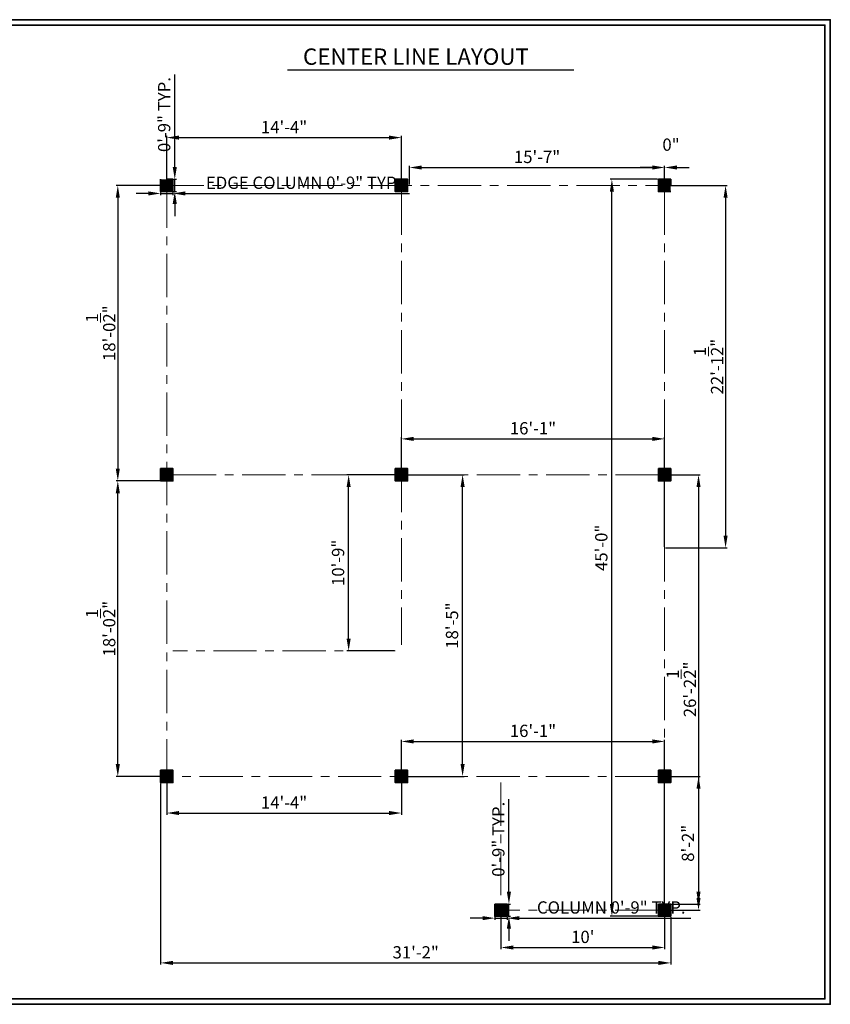
# Model space of a CAD drawing. Units: inches. Extents: x 2396 to 4051, y 1419 to 2191.
# Tile 7 of 7: x 3457 to 4051, y 1470 to 2191. Entities that reach past the tile are written whole.
import ezdxf

# ---------------------------------------------------------------- set-up
doc = ezdxf.new("R2010")
doc.units = ezdxf.units.IN
doc.linetypes.add('CENTER', pattern=[50.8, 31.75, -6.35, 6.35, -6.35])
for name, color, linetype, lineweight in [('A-ANNO-TITL', 7, 'Continuous', 25), ('A-ANNO-TTLB', 7, 'Continuous', 35), ('S-ANNO-DIMS', 2, 'Continuous', 18), ('S-GRID', 1, 'CENTER', 18)]:
    doc.layers.add(name, color=color, linetype=linetype, lineweight=lineweight)
doc.layers.add('S-COLS', color=242, linetype='Continuous', lineweight=35, true_color=0xcd2027)
doc.styles.get("Standard").update_dxf_attribs({"font": 'arial.ttf'})
doc.dimstyles.new('ISO-25', dxfattribs={"dimtxt": 9, "dimasz": 9, "dimexe": 1.25, "dimexo": 0.625, "dimgap": 2, "dimtad": 1, "dimdec": 1, "dimlunit": 4, "dimtxsty": 'Standard', "dimcen": 2.5, "dimadec": 0, "dimazin": 0, "dimtfac": 1, "dimtdec": 1, "dimtmove": 0, "dimatfit": 3, "dimfxl": 1, "dimarcsym": 0})

# ---------------------------------------------------------------- blocks, each defined once
blk = doc.blocks.new('*D15')
at = {"layer": 'Defpoints', "color": 0, "transparency": 16777216}
for p in [(3736.71, 2104.86), (3564.71, 2069.8), (3736.71, 2069.8)]:
    blk.add_point(p, dxfattribs=at)
at = {"layer": 'S-ANNO-DIMS', "color": 0, "lineweight": -2, "transparency": 16777216}
for p, q in [((3564.71, 2070.43), (3564.71, 2106.11)), ((3573.71, 2104.86), (3727.71, 2104.86)), ((3736.71, 2070.43), (3736.71, 2106.11))]:
    blk.add_line(p, q, dxfattribs=at)
at = {"layer": 'S-ANNO-DIMS', "color": 0, "transparency": 16777216}
for points in [[(3573.71, 2106.36), (3573.71, 2103.36), (3564.71, 2104.86)], [(3727.71, 2106.36), (3727.71, 2103.36), (3736.71, 2104.86)]]:
    blk.add_solid(points, dxfattribs=at)
at = {"layer": 'S-ANNO-DIMS', "color": 0, "transparency": 16777216, "insert": (3650.71, 2111.38), "char_height": 9, "attachment_point": 5}
blk.add_mtext('14\'-4"', dxfattribs=at)
blk = doc.blocks.new('*D16')
at = {"layer": 'Defpoints', "color": 0, "transparency": 16777216}
for p in [(3929.71, 2082.95), (3742.71, 2069.8), (3929.71, 2069.8)]:
    blk.add_point(p, dxfattribs=at)
at = {"layer": 'S-ANNO-DIMS', "color": 0, "lineweight": -2, "transparency": 16777216}
for p, q in [((3742.71, 2070.43), (3742.71, 2084.2)), ((3751.71, 2082.95), (3920.71, 2082.95)), ((3929.71, 2070.43), (3929.71, 2084.2))]:
    blk.add_line(p, q, dxfattribs=at)
at = {"layer": 'S-ANNO-DIMS', "color": 0, "transparency": 16777216}
for points in [[(3751.71, 2084.45), (3751.71, 2081.45), (3742.71, 2082.95)], [(3920.71, 2084.45), (3920.71, 2081.45), (3929.71, 2082.95)]]:
    blk.add_solid(points, dxfattribs=at)
at = {"layer": 'S-ANNO-DIMS', "color": 0, "transparency": 16777216, "insert": (3836.21, 2089.54), "char_height": 9, "attachment_point": 5}
blk.add_mtext('15\'-7"', dxfattribs=at)
blk = doc.blocks.new('*D17')
at = {"layer": 'Defpoints', "color": 0, "transparency": 16777216}
for p in [(3929.71, 2082.95), (3929.71, 2082.95), (3929.71, 2069.8)]:
    blk.add_point(p, dxfattribs=at)
at = {"layer": 'S-ANNO-DIMS', "color": 0, "lineweight": -2, "transparency": 16777216}
for p, q in [((3920.71, 2082.95), (3911.71, 2082.95)), ((3929.71, 2070.43), (3929.71, 2084.2)), ((3929.71, 2083.57), (3929.71, 2084.2)), ((3938.71, 2082.95), (3947.71, 2082.95))]:
    blk.add_line(p, q, dxfattribs=at)
at = {"layer": 'S-ANNO-DIMS', "color": 0, "transparency": 16777216}
for points in [[(3920.71, 2084.45), (3920.71, 2081.45), (3929.71, 2082.95)], [(3938.71, 2084.45), (3938.71, 2081.45), (3929.71, 2082.95)]]:
    blk.add_solid(points, dxfattribs=at)
at = {"layer": 'S-ANNO-DIMS', "color": 0, "transparency": 16777216, "insert": (3934.41, 2098.54), "char_height": 9, "attachment_point": 5}
blk.add_mtext('0"', dxfattribs=at)
blk = doc.blocks.new('*D18')
at = {"layer": 'Defpoints', "color": 0, "transparency": 16777216}
for p in [(3564.71, 2069.8), (3528.81, 1853.3), (3564.71, 1853.3)]:
    blk.add_point(p, dxfattribs=at)
at = {"layer": 'S-ANNO-DIMS', "color": 0, "lineweight": -2, "transparency": 16777216}
for p, q in [((3564.09, 2069.8), (3527.56, 2069.8)), ((3528.81, 2060.8), (3528.81, 1862.3)), ((3564.09, 1853.3), (3527.56, 1853.3))]:
    blk.add_line(p, q, dxfattribs=at)
at = {"layer": 'S-ANNO-DIMS', "color": 0, "transparency": 16777216}
for points in [[(3527.31, 2060.8), (3530.31, 2060.8), (3528.81, 2069.8)], [(3527.31, 1862.3), (3530.31, 1862.3), (3528.81, 1853.3)]]:
    blk.add_solid(points, dxfattribs=at)
at = {"layer": 'S-ANNO-DIMS', "color": 0, "transparency": 16777216, "insert": (3516.2, 1961.55), "char_height": 9, "attachment_point": 5, "rotation": 90}
blk.add_mtext('18\'-0{\\H1x;\\S1/2;}"', dxfattribs=at)
blk = doc.blocks.new('*D19')
at = {"layer": 'Defpoints', "color": 0, "transparency": 16777216}
for p in [(3528.81, 1853.3), (3564.71, 1853.3), (3564.71, 1636.8)]:
    blk.add_point(p, dxfattribs=at)
at = {"layer": 'S-ANNO-DIMS', "color": 0, "lineweight": -2, "transparency": 16777216}
for p, q in [((3564.09, 1853.3), (3527.56, 1853.3)), ((3528.81, 1645.8), (3528.81, 1844.3)), ((3564.09, 1636.8), (3527.56, 1636.8))]:
    blk.add_line(p, q, dxfattribs=at)
at = {"layer": 'S-ANNO-DIMS', "color": 0, "transparency": 16777216}
for points in [[(3527.31, 1844.3), (3530.31, 1844.3), (3528.81, 1853.3)], [(3527.31, 1645.8), (3530.31, 1645.8), (3528.81, 1636.8)]]:
    blk.add_solid(points, dxfattribs=at)
at = {"layer": 'S-ANNO-DIMS', "color": 0, "transparency": 16777216, "insert": (3516.2, 1745.05), "char_height": 9, "attachment_point": 5, "rotation": 90}
blk.add_mtext('18\'-0{\\H1x;\\S1/2;}"', dxfattribs=at)
blk = doc.blocks.new('*D20')
at = {"layer": 'Defpoints', "color": 0, "transparency": 16777216}
for p in [(3564.71, 1632.3), (3736.71, 1636.8), (3736.71, 1609.97)]:
    blk.add_point(p, dxfattribs=at)
at = {"layer": 'S-ANNO-DIMS', "color": 0, "lineweight": -2, "transparency": 16777216}
for p, q in [((3564.71, 1631.68), (3564.71, 1608.72)), ((3736.71, 1636.18), (3736.71, 1608.72)), ((3573.71, 1609.97), (3727.71, 1609.97))]:
    blk.add_line(p, q, dxfattribs=at)
at = {"layer": 'S-ANNO-DIMS', "color": 0, "transparency": 16777216}
for points in [[(3573.71, 1611.47), (3573.71, 1608.47), (3564.71, 1609.97)], [(3727.71, 1611.47), (3727.71, 1608.47), (3736.71, 1609.97)]]:
    blk.add_solid(points, dxfattribs=at)
at = {"layer": 'S-ANNO-DIMS', "color": 0, "transparency": 16777216, "insert": (3650.71, 1616.49), "char_height": 9, "attachment_point": 5}
blk.add_mtext('14\'-4"', dxfattribs=at)
blk = doc.blocks.new('*D21')
at = {"layer": 'Defpoints', "color": 0, "transparency": 16777216}
for p in [(3929.71, 1662.41), (3736.71, 1636.8), (3929.71, 1543.3)]:
    blk.add_point(p, dxfattribs=at)
at = {"layer": 'S-ANNO-DIMS', "color": 0, "lineweight": -2, "transparency": 16777216}
for p, q in [((3736.71, 1637.43), (3736.71, 1663.66)), ((3745.71, 1662.41), (3920.71, 1662.41)), ((3929.71, 1543.93), (3929.71, 1663.66))]:
    blk.add_line(p, q, dxfattribs=at)
at = {"layer": 'S-ANNO-DIMS', "color": 0, "transparency": 16777216}
for points in [[(3745.71, 1663.91), (3745.71, 1660.91), (3736.71, 1662.41)], [(3920.71, 1663.91), (3920.71, 1660.91), (3929.71, 1662.41)]]:
    blk.add_solid(points, dxfattribs=at)
at = {"layer": 'S-ANNO-DIMS', "color": 0, "transparency": 16777216, "insert": (3833.21, 1669), "char_height": 9, "attachment_point": 5}
blk.add_mtext('16\'-1"', dxfattribs=at)
blk = doc.blocks.new('*D22')
at = {"layer": 'Defpoints', "color": 0, "transparency": 16777216}
for p in [(3929.71, 1636.8), (3929.71, 1538.8), (3954.57, 1538.8)]:
    blk.add_point(p, dxfattribs=at)
at = {"layer": 'S-ANNO-DIMS', "color": 0, "lineweight": -2, "transparency": 16777216}
for p, q in [((3930.34, 1636.8), (3955.82, 1636.8)), ((3954.57, 1627.8), (3954.57, 1547.8)), ((3930.34, 1538.8), (3955.82, 1538.8))]:
    blk.add_line(p, q, dxfattribs=at)
at = {"layer": 'S-ANNO-DIMS', "color": 0, "transparency": 16777216}
for points in [[(3953.07, 1627.8), (3956.07, 1627.8), (3954.57, 1636.8)], [(3953.07, 1547.8), (3956.07, 1547.8), (3954.57, 1538.8)]]:
    blk.add_solid(points, dxfattribs=at)
at = {"layer": 'S-ANNO-DIMS', "color": 0, "transparency": 16777216, "insert": (3947.97, 1587.8), "char_height": 9, "attachment_point": 5, "rotation": 90}
blk.add_mtext('8\'-2"', dxfattribs=at)
blk = doc.blocks.new('*D23')
at = {"layer": 'Defpoints', "color": 0, "transparency": 16777216}
for p in [(3809.71, 1538.8), (3929.71, 1538.8), (3929.71, 1511.44)]:
    blk.add_point(p, dxfattribs=at)
at = {"layer": 'S-ANNO-DIMS', "color": 0, "lineweight": -2, "transparency": 16777216}
for p, q in [((3809.71, 1538.18), (3809.71, 1510.19)), ((3929.71, 1538.18), (3929.71, 1510.19)), ((3818.71, 1511.44), (3920.71, 1511.44))]:
    blk.add_line(p, q, dxfattribs=at)
at = {"layer": 'S-ANNO-DIMS', "color": 0, "transparency": 16777216}
for points in [[(3818.71, 1512.94), (3818.71, 1509.94), (3809.71, 1511.44)], [(3920.71, 1512.94), (3920.71, 1509.94), (3929.71, 1511.44)]]:
    blk.add_solid(points, dxfattribs=at)
at = {"layer": 'S-ANNO-DIMS', "color": 0, "transparency": 16777216, "insert": (3869.71, 1518.04), "char_height": 9, "attachment_point": 5}
blk.add_mtext("10'", dxfattribs=at)
blk = doc.blocks.new('*D24')
at = {"layer": 'Defpoints', "color": 0, "transparency": 16777216}
for p in [(3929.71, 2069.8), (3929.71, 1804.3), (3974.42, 1804.3)]:
    blk.add_point(p, dxfattribs=at)
at = {"layer": 'S-ANNO-DIMS', "color": 0, "lineweight": -2, "transparency": 16777216}
for p, q in [((3930.34, 2069.8), (3975.67, 2069.8)), ((3974.42, 2060.8), (3974.42, 1813.3)), ((3930.34, 1804.3), (3975.67, 1804.3))]:
    blk.add_line(p, q, dxfattribs=at)
at = {"layer": 'S-ANNO-DIMS', "color": 0, "transparency": 16777216}
for points in [[(3972.92, 2060.8), (3975.92, 2060.8), (3974.42, 2069.8)], [(3972.92, 1813.3), (3975.92, 1813.3), (3974.42, 1804.3)]]:
    blk.add_solid(points, dxfattribs=at)
at = {"layer": 'S-ANNO-DIMS', "color": 0, "transparency": 16777216, "insert": (3961.89, 1937.05), "char_height": 9, "attachment_point": 5, "rotation": 90}
blk.add_mtext('22\'-1{\\H1x;\\S1/2;}"', dxfattribs=at)
blk = doc.blocks.new('*D25')
at = {"layer": 'Defpoints', "color": 0, "transparency": 16777216}
for p in [(3929.71, 1857.8), (3929.71, 1543.3), (3954.57, 1543.3)]:
    blk.add_point(p, dxfattribs=at)
at = {"layer": 'S-ANNO-DIMS', "color": 0, "lineweight": -2, "transparency": 16777216}
for p, q in [((3930.34, 1857.8), (3955.82, 1857.8)), ((3954.57, 1848.8), (3954.57, 1552.3)), ((3930.34, 1543.3), (3955.82, 1543.3))]:
    blk.add_line(p, q, dxfattribs=at)
at = {"layer": 'S-ANNO-DIMS', "color": 0, "transparency": 16777216}
for points in [[(3953.07, 1848.8), (3956.07, 1848.8), (3954.57, 1857.8)], [(3953.07, 1552.3), (3956.07, 1552.3), (3954.57, 1543.3)]]:
    blk.add_solid(points, dxfattribs=at)
at = {"layer": 'S-ANNO-DIMS', "color": 0, "transparency": 16777216, "insert": (3941.95, 1700.55), "char_height": 9, "attachment_point": 5, "rotation": 90}
blk.add_mtext('26\'-2{\\H1x;\\S1/2;}"', dxfattribs=at)
blk = doc.blocks.new('*D26')
at = {"layer": 'Defpoints', "color": 0, "transparency": 16777216}
for p in [(3929.71, 1884.11), (3736.71, 1857.8), (3929.71, 1804.3)]:
    blk.add_point(p, dxfattribs=at)
at = {"layer": 'S-ANNO-DIMS', "color": 0, "lineweight": -2, "transparency": 16777216}
for p, q in [((3736.71, 1858.43), (3736.71, 1885.36)), ((3745.71, 1884.11), (3920.71, 1884.11)), ((3929.71, 1804.93), (3929.71, 1885.36))]:
    blk.add_line(p, q, dxfattribs=at)
at = {"layer": 'S-ANNO-DIMS', "color": 0, "transparency": 16777216}
for points in [[(3745.71, 1885.61), (3745.71, 1882.61), (3736.71, 1884.11)], [(3920.71, 1885.61), (3920.71, 1882.61), (3929.71, 1884.11)]]:
    blk.add_solid(points, dxfattribs=at)
at = {"layer": 'S-ANNO-DIMS', "color": 0, "transparency": 16777216, "insert": (3833.21, 1890.71), "char_height": 9, "attachment_point": 5}
blk.add_mtext('16\'-1"', dxfattribs=at)
blk = doc.blocks.new('*D27')
at = {"layer": 'Defpoints', "color": 0, "transparency": 16777216}
for p in [(3736.71, 1857.8), (3781.61, 1857.8), (3736.71, 1636.8)]:
    blk.add_point(p, dxfattribs=at)
at = {"layer": 'S-ANNO-DIMS', "color": 0, "lineweight": -2, "transparency": 16777216}
for p, q in [((3737.34, 1857.8), (3782.86, 1857.8)), ((3781.61, 1645.8), (3781.61, 1848.8)), ((3737.34, 1636.8), (3782.86, 1636.8))]:
    blk.add_line(p, q, dxfattribs=at)
at = {"layer": 'S-ANNO-DIMS', "color": 0, "transparency": 16777216}
for points in [[(3780.11, 1848.8), (3783.11, 1848.8), (3781.61, 1857.8)], [(3780.11, 1645.8), (3783.11, 1645.8), (3781.61, 1636.8)]]:
    blk.add_solid(points, dxfattribs=at)
at = {"layer": 'S-ANNO-DIMS', "color": 0, "transparency": 16777216, "insert": (3775.01, 1747.3), "char_height": 9, "attachment_point": 5, "rotation": 90}
blk.add_mtext('18\'-5"', dxfattribs=at)
blk = doc.blocks.new('COL-9X9')
h = blk.add_hatch(color=256)
h.dxf.hatch_style = 1
h.paths.add_polyline_path([(9, 9), (0, 9), (0, 0), (9, 0)])
blk.add_lwpolyline([(0, 9), (9, 9), (9, 0), (0, 0)], close=True)
blk = doc.blocks.new('COL-9X9-EDGE-NODE')
h = blk.add_hatch(color=256)
h.dxf.hatch_style = 1
h.paths.add_polyline_path([(0, 0), (9, 0), (9, 9), (0, 9)])
blk.add_lwpolyline([(4.5, 9), (9, 9), (9, 0), (0, 0), (0, 9)])
blk = doc.blocks.new('*D36')
at = {"layer": 'Defpoints', "color": 0, "transparency": 16777216}
for p in [(3805.21, 1534.3), (3814.21, 1534.3), (3814.21, 1532.95)]:
    blk.add_point(p, dxfattribs=at)
at = {"layer": 'S-ANNO-DIMS', "color": 0, "lineweight": -2, "transparency": 16777216}
for p, q in [((3796.21, 1532.95), (3787.21, 1532.95)), ((3805.21, 1533.68), (3805.21, 1531.7)), ((3805.21, 1532.95), (3814.21, 1532.95)), ((3814.21, 1533.68), (3814.21, 1531.7)), ((3823.21, 1532.95), (3948.95, 1532.95))]:
    blk.add_line(p, q, dxfattribs=at)
at = {"layer": 'S-ANNO-DIMS', "color": 0, "transparency": 16777216}
for points in [[(3796.21, 1534.45), (3796.21, 1531.45), (3805.21, 1532.95)], [(3823.21, 1534.45), (3823.21, 1531.45), (3814.21, 1532.95)]]:
    blk.add_solid(points, dxfattribs=at)
at = {"layer": 'S-ANNO-DIMS', "color": 0, "transparency": 16777216, "insert": (3890.58, 1539.61), "char_height": 9, "attachment_point": 5}
blk.add_mtext('COLUMN 0\'-9" TYP.', dxfattribs=at)
blk = doc.blocks.new('*D37')
at = {"layer": 'Defpoints', "color": 0, "transparency": 16777216}
for p in [(3814.21, 1543.3), (3815.56, 1543.3), (3814.21, 1534.3)]:
    blk.add_point(p, dxfattribs=at)
at = {"layer": 'S-ANNO-DIMS', "color": 0, "lineweight": -2, "transparency": 16777216}
for p, q in [((3815.56, 1552.3), (3815.56, 1620.16)), ((3814.84, 1543.3), (3816.81, 1543.3)), ((3815.56, 1534.3), (3815.56, 1543.3)), ((3814.84, 1534.3), (3816.81, 1534.3)), ((3815.56, 1525.3), (3815.56, 1516.3))]:
    blk.add_line(p, q, dxfattribs=at)
at = {"layer": 'S-ANNO-DIMS', "color": 0, "transparency": 16777216}
for points in [[(3814.06, 1552.3), (3817.06, 1552.3), (3815.56, 1543.3)], [(3814.06, 1525.3), (3817.06, 1525.3), (3815.56, 1534.3)]]:
    blk.add_solid(points, dxfattribs=at)
at = {"layer": 'S-ANNO-DIMS', "color": 0, "transparency": 16777216, "insert": (3808.97, 1590.73), "char_height": 9, "attachment_point": 5, "rotation": 90}
blk.add_mtext('0\'-9" TYP.', dxfattribs=at)
blk = doc.blocks.new('*D38')
at = {"layer": 'Defpoints', "color": 0, "transparency": 16777216}
for p in [(3560.21, 2065.3), (3569.21, 2065.3), (3569.21, 2063.95)]:
    blk.add_point(p, dxfattribs=at)
at = {"layer": 'S-ANNO-DIMS', "color": 0, "lineweight": -2, "transparency": 16777216}
for p, q in [((3551.21, 2063.95), (3542.21, 2063.95)), ((3560.21, 2064.68), (3560.21, 2062.7)), ((3560.21, 2063.95), (3569.21, 2063.95)), ((3569.21, 2064.68), (3569.21, 2062.7)), ((3578.21, 2063.95), (3742.7, 2063.95))]:
    blk.add_line(p, q, dxfattribs=at)
at = {"layer": 'S-ANNO-DIMS', "color": 0, "transparency": 16777216}
for points in [[(3551.21, 2065.45), (3551.21, 2062.45), (3560.21, 2063.95)], [(3578.21, 2065.45), (3578.21, 2062.45), (3569.21, 2063.95)]]:
    blk.add_solid(points, dxfattribs=at)
at = {"layer": 'S-ANNO-DIMS', "color": 0, "transparency": 16777216, "insert": (3664.96, 2070.61), "char_height": 9, "attachment_point": 5}
blk.add_mtext('EDGE COLUMN 0\'-9" TYP.', dxfattribs=at)
blk = doc.blocks.new('*D39')
at = {"layer": 'Defpoints', "color": 0, "transparency": 16777216}
for p in [(3569.21, 2074.3), (3570.56, 2074.3), (3569.21, 2065.3)]:
    blk.add_point(p, dxfattribs=at)
at = {"layer": 'S-ANNO-DIMS', "color": 0, "lineweight": -2, "transparency": 16777216}
for p, q in [((3570.56, 2083.3), (3570.56, 2151.16)), ((3569.84, 2074.3), (3571.81, 2074.3)), ((3570.56, 2065.3), (3570.56, 2074.3)), ((3569.84, 2065.3), (3571.81, 2065.3)), ((3570.56, 2056.3), (3570.56, 2047.3))]:
    blk.add_line(p, q, dxfattribs=at)
at = {"layer": 'S-ANNO-DIMS', "color": 0, "transparency": 16777216}
for points in [[(3569.06, 2083.3), (3572.06, 2083.3), (3570.56, 2074.3)], [(3569.06, 2056.3), (3572.06, 2056.3), (3570.56, 2065.3)]]:
    blk.add_solid(points, dxfattribs=at)
at = {"layer": 'S-ANNO-DIMS', "color": 0, "transparency": 16777216, "insert": (3563.97, 2121.73), "char_height": 9, "attachment_point": 5, "rotation": 90}
blk.add_mtext('0\'-9" TYP.', dxfattribs=at)
blk = doc.blocks.new('*D109')
at = {"layer": 'Defpoints', "color": 0, "transparency": 16777216}
for p in [(3560.21, 1632.3), (3934.21, 1534.3), (3934.21, 1500.15)]:
    blk.add_point(p, dxfattribs=at)
at = {"layer": 'S-ANNO-DIMS', "color": 0, "lineweight": -2, "transparency": 16777216}
for p, q in [((3560.21, 1631.68), (3560.21, 1498.9)), ((3934.21, 1533.68), (3934.21, 1498.9)), ((3569.21, 1500.15), (3925.21, 1500.15))]:
    blk.add_line(p, q, dxfattribs=at)
at = {"layer": 'S-ANNO-DIMS', "color": 0, "transparency": 16777216}
for points in [[(3569.21, 1501.65), (3569.21, 1498.65), (3560.21, 1500.15)], [(3925.21, 1501.65), (3925.21, 1498.65), (3934.21, 1500.15)]]:
    blk.add_solid(points, dxfattribs=at)
at = {"layer": 'S-ANNO-DIMS', "color": 0, "transparency": 16777216, "insert": (3747.21, 1506.75), "char_height": 9, "attachment_point": 5}
blk.add_mtext('31\'-2"', dxfattribs=at)
blk = doc.blocks.new('*D110')
at = {"layer": 'Defpoints', "color": 0, "transparency": 16777216}
for p in [(3891.06, 2074.3), (3925.21, 2074.3), (3925.21, 1534.3)]:
    blk.add_point(p, dxfattribs=at)
at = {"layer": 'S-ANNO-DIMS', "color": 0, "lineweight": -2, "transparency": 16777216}
for p, q in [((3924.59, 2074.3), (3889.81, 2074.3)), ((3891.06, 1543.3), (3891.06, 2065.3)), ((3924.59, 1534.3), (3889.81, 1534.3))]:
    blk.add_line(p, q, dxfattribs=at)
at = {"layer": 'S-ANNO-DIMS', "color": 0, "transparency": 16777216}
for points in [[(3889.56, 2065.3), (3892.56, 2065.3), (3891.06, 2074.3)], [(3889.56, 1543.3), (3892.56, 1543.3), (3891.06, 1534.3)]]:
    blk.add_solid(points, dxfattribs=at)
at = {"layer": 'S-ANNO-DIMS', "color": 0, "transparency": 16777216, "insert": (3884.47, 1804.3), "char_height": 9, "attachment_point": 5, "rotation": 90}
blk.add_mtext('45\'-0"', dxfattribs=at)
blk = doc.blocks.new('*D111')
at = {"layer": 'Defpoints', "color": 0, "transparency": 16777216}
for p in [(3698.06, 1857.8), (3732.21, 1857.8), (3732.21, 1728.8)]:
    blk.add_point(p, dxfattribs=at)
at = {"layer": 'S-ANNO-DIMS', "color": 0, "lineweight": -2, "transparency": 16777216}
for p, q in [((3731.59, 1857.8), (3696.81, 1857.8)), ((3698.06, 1737.8), (3698.06, 1848.8)), ((3731.59, 1728.8), (3696.81, 1728.8))]:
    blk.add_line(p, q, dxfattribs=at)
at = {"layer": 'S-ANNO-DIMS', "color": 0, "transparency": 16777216}
for points in [[(3696.56, 1848.8), (3699.56, 1848.8), (3698.06, 1857.8)], [(3696.56, 1737.8), (3699.56, 1737.8), (3698.06, 1728.8)]]:
    blk.add_solid(points, dxfattribs=at)
at = {"layer": 'S-ANNO-DIMS', "color": 0, "transparency": 16777216, "insert": (3691.47, 1793.3), "char_height": 9, "attachment_point": 5, "rotation": 90}
blk.add_mtext('10\'-9"', dxfattribs=at)

msp = doc.modelspace()

# ---------------------------------------------------------------- linework, layer by layer
at = {"layer": 'A-ANNO-TITL'}
msp.add_line((3653.21, 2154.51), (3863.24, 2154.51), dxfattribs=at)
at = {"layer": 'A-ANNO-TTLB'}
for points in [[(2460.66, 2191.26), (4051.21, 2191.26), (4051.21, 1469.82), (2460.66, 1469.82)], [(2464.66, 2187.26), (4047.21, 2187.26), (4047.21, 1473.82), (2464.66, 1473.82)]]:
    msp.add_lwpolyline(points, close=True, dxfattribs=at)
at = {"layer": 'S-COLS'}
msp.add_line((3560.21, 1853.3), (3560.21, 1862.3), dxfattribs=at)
at = {"layer": 'S-GRID'}
for p, q in [((3564.71, 1632.3), (3564.71, 2074.3)), ((3560.21, 2069.8), (3925.21, 2069.8)), ((3736.71, 2065.3), (3736.71, 1733.3)), ((3929.71, 2065.3), (3929.71, 1543.3)), ((3569.21, 1857.8), (3732.21, 1857.8)), ((3741.21, 1857.8), (3925.21, 1857.8)), ((3732.21, 1728.8), (3569.21, 1728.8)), ((3925.21, 1636.8), (3569.21, 1636.8)), ((3809.71, 1632.3), (3809.71, 1543.3)), ((3925.21, 1538.8), (3814.21, 1538.8))]:
    msp.add_line(p, q, dxfattribs=at)

# ---------------------------------------------------------------- block references
at = {"layer": 'S-COLS'}
for name, p in [('COL-9X9-EDGE-NODE', (3560.21, 2065.3)), ('COL-9X9', (3732.21, 2065.3)), ('COL-9X9', (3560.21, 1853.3)), ('COL-9X9', (3732.21, 1853.3)), ('COL-9X9', (3925.21, 1853.3)), ('COL-9X9', (3560.21, 1632.3)), ('COL-9X9', (3732.21, 1632.3)), ('COL-9X9', (3925.21, 1632.3)), ('COL-9X9', (3805.21, 1534.3)), ('COL-9X9', (3925.21, 1534.3))]:
    msp.add_blockref(name, p, dxfattribs=at)
at = {"layer": 'S-COLS', "extrusion": (0, 0, -1), "zscale": -1, "rotation": 89.99999999999162}
msp.add_blockref('COL-9X9-EDGE-NODE', (-3925.21, 2065.3), dxfattribs=at)

# ---------------------------------------------------------------- texts
at = {"layer": 'A-ANNO-TITL', "insert": (3664.59, 2170.19), "char_height": 12, "attachment_point": 1}
msp.add_mtext_dynamic_manual_height_columns('{\\fArial|b1|i0|c0|p34;CENTER LINE LAYOUT}', width=349.2365, gutter_width=12.5, heights=[0], dxfattribs=at)

# ---------------------------------------------------------------- dimensions: what is measured, and where the dimension line sits
at = {"layer": 'S-ANNO-DIMS'}
for base, p1, p2, picture, middle in [((3570.56, 2074.3), (3569.21, 2065.3), (3569.21, 2074.3), '*D39', (3563.97, 2121.73)), ((3815.56, 1543.3), (3814.21, 1534.3), (3814.21, 1543.3), '*D37', (3808.97, 1590.73))]:
    dim = msp.add_linear_dim(base=base, p1=p1, p2=p2, angle=90, text='<> TYP.', dimstyle='ISO-25', override={"dimdec": 1, "dimlfac": 1, "dimrnd": 0, "dimzin": 1, "dimdsep": 46, "dimlunit": 4, "dimfrac": 2}, dxfattribs=at)
    dim.commit()
    dim.dimension.update_dxf_attribs({"geometry": picture, "text_midpoint": middle})
dim = msp.add_linear_dim(base=(3736.71, 2104.86), p1=(3564.71, 2069.8), p2=(3736.71, 2069.8), dimstyle='ISO-25', override={"dimclrd": 0, "dimclre": 0, "dimclrt": 0}, dxfattribs=at)
dim.commit()
dim.dimension.update_dxf_attribs({"geometry": '*D15', "text_midpoint": (3650.71, 2104.86), "dimtype": 160})
for base, p1, p2, override, picture, middle in [((3929.71447039, 2082.94780016), (3929.71447039, 2069.80064987), (3929.71447039, 2082.94780016), {"dimclrd": 0, "dimclre": 0, "dimclrt": 0, "dimtmove": 1}, '*D17', (3934.41447039, 2098.54295705)), ((3929.71, 2082.95), (3742.71, 2069.8), (3929.71, 2069.8), {"dimclrd": 0, "dimclre": 0, "dimclrt": 0, "dimtmove": 1}, '*D16', (3836.21, 2089.54)), ((3929.71, 1884.11), (3736.71, 1857.8), (3929.71, 1804.3), {"dimclrd": 0, "dimclre": 0, "dimclrt": 0}, '*D26', (3833.21, 1890.71)), ((3929.71, 1662.41), (3736.71, 1636.8), (3929.71, 1543.3), {"dimclrd": 0, "dimclre": 0, "dimclrt": 0}, '*D21', (3833.21, 1669)), ((3934.21, 1500.15), (3560.21, 1632.3), (3934.21, 1534.3), {"dimdec": 1, "dimlfac": 1, "dimrnd": 0, "dimzin": 1, "dimdsep": 46, "dimlunit": 4, "dimfrac": 2}, '*D109', (3747.21, 1506.75)), ((3736.71, 1609.97), (3564.71, 1632.3), (3736.71, 1636.8), {"dimclrd": 0, "dimclre": 0, "dimclrt": 0}, '*D20', (3650.71, 1616.49)), ((3929.71, 1511.44), (3809.71, 1538.8), (3929.71, 1538.8), {"dimclrd": 0, "dimclre": 0, "dimclrt": 0}, '*D23', (3869.71, 1518.04))]:
    dim = msp.add_linear_dim(base=base, p1=p1, p2=p2, dimstyle='ISO-25', override=override, dxfattribs=at)
    dim.commit()
    dim.dimension.update_dxf_attribs({"geometry": picture, "text_midpoint": middle})
for base, p1, p2, text, picture, middle in [((3569.21, 2063.95), (3560.21, 2065.3), (3569.21, 2065.3), 'EDGE COLUMN <> TYP.', '*D38', (3664.96, 2070.61)), ((3814.21, 1532.95), (3805.21, 1534.3), (3814.21, 1534.3), 'COLUMN <> TYP.', '*D36', (3890.58, 1539.61))]:
    dim = msp.add_linear_dim(base=base, p1=p1, p2=p2, text=text, dimstyle='ISO-25', override={"dimdec": 1, "dimlfac": 1, "dimrnd": 0, "dimzin": 1, "dimdsep": 46, "dimlunit": 4, "dimfrac": 2}, dxfattribs=at)
    dim.commit()
    dim.dimension.update_dxf_attribs({"geometry": picture, "text_midpoint": middle})
for base, p1, p2, override, picture, middle in [((3891.06, 2074.3), (3925.21, 1534.3), (3925.21, 2074.3), {"dimdec": 1, "dimlfac": 1, "dimrnd": 0, "dimzin": 1, "dimdsep": 46, "dimlunit": 4, "dimfrac": 2}, '*D110', (3884.47, 1804.3)), ((3528.81, 1853.3), (3564.71, 2069.8), (3564.71, 1853.3), {"dimclrd": 0, "dimclre": 0, "dimclrt": 0}, '*D18', (3516.2, 1961.55)), ((3974.42, 1804.3), (3929.71, 2069.8), (3929.71, 1804.3), {"dimclrd": 0, "dimclre": 0, "dimclrt": 0}, '*D24', (3961.89, 1937.05)), ((3698.06, 1857.8), (3732.21, 1728.8), (3732.21, 1857.8), {"dimdec": 1, "dimlfac": 1, "dimrnd": 0, "dimzin": 1, "dimdsep": 46, "dimlunit": 4, "dimfrac": 2}, '*D111', (3691.47, 1793.3)), ((3954.57, 1543.3), (3929.71, 1857.8), (3929.71, 1543.3), {"dimclrd": 0, "dimclre": 0, "dimclrt": 0}, '*D25', (3941.95, 1700.55)), ((3528.81, 1853.3), (3564.71, 1636.8), (3564.71, 1853.3), {"dimclrd": 0, "dimclre": 0, "dimclrt": 0}, '*D19', (3516.2, 1745.05)), ((3954.57, 1538.8), (3929.71, 1636.8), (3929.71, 1538.8), {"dimclrd": 0, "dimclre": 0, "dimclrt": 0}, '*D22', (3947.97, 1587.8))]:
    dim = msp.add_linear_dim(base=base, p1=p1, p2=p2, angle=90, dimstyle='ISO-25', override=override, dxfattribs=at)
    dim.commit()
    dim.dimension.update_dxf_attribs({"geometry": picture, "text_midpoint": middle})
dim = msp.add_linear_dim(base=(3781.61, 1857.8), p1=(3736.71, 1636.8), p2=(3736.71, 1857.8), angle=90, dimstyle='ISO-25', override={"dimclrd": 0, "dimclre": 0, "dimclrt": 0}, dxfattribs=at)
dim.commit()
dim.dimension.update_dxf_attribs({"geometry": '*D27', "text_midpoint": (3781.61, 1747.3), "dimtype": 160})

doc.saveas('drawing.dxf')
